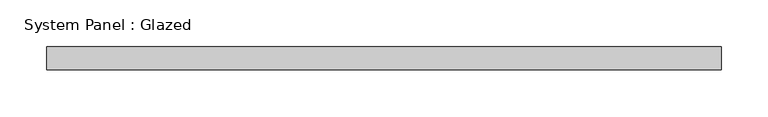
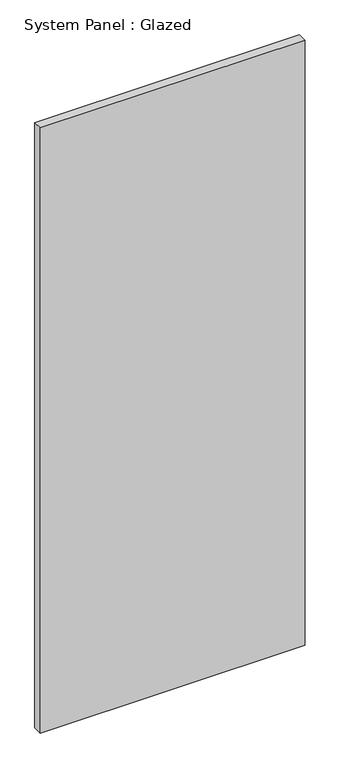
"""IFC4 building model written with IfcOpenShell, lengths in millimetres: plate geometry, System Panel : Glazed."""

from ifc_helpers import new_model, si_unit, origin, origin_with_axes, place, context, project, spatial, polyline, outline, extrude, source, transform, mapped, element, save


def system_panel_glazed_3b80f955(model_context):
    return source(origin(), model_context, "Body", "SweptSolid", [
        extrude(outline(polyline([(362.5, 24.5), (-362.5, 24.5), (-362.5, 49.5), (362.5, 49.5), (362.5, 24.5)])), origin_with_axes(), (0.0, 0.0, 1.0), 1750.0),
    ])


if __name__ == "__main__":
    model = new_model("IFC4")
    model_context = context("Model", 3, world=origin())
    ifc_project = project(units=[si_unit("LENGTHUNIT", "METRE", prefix="MILLI")], contexts=[model_context])
    site = spatial("IfcSite", under=ifc_project)
    building = spatial("IfcBuilding", under=site)
    placement = place(None, origin())
    system_panel_glazed_shape = system_panel_glazed_3b80f955(model_context)
    element("IfcPlate", 1, ObjectType="System Panel : Glazed", at=placement, inside=building, context=model_context, shape_type="MappedRepresentation", body=[
        mapped(system_panel_glazed_shape, transform((0.0, 0.0, 0.0), x_axis=(1.0, 0.0, 0.0), y_axis=(0.0, 1.0, 0.0), z_axis=(0.0, 0.0, 1.0))),
    ])
    save(model, "model.ifc")

# Revit data of these elements
# Type "System Panel : Glazed"
#   Construction Type Id = "GSP4R"
#   Analytic Construction = "1/8 in Pilkington single glazing"
#   Visual Light Transmittance = 0.9
#   Solar Heat Gain Coefficient = 0.86
#   Heat Transfer Coefficient (U) = 6.7069 W/(m²·K)
#   Define Thermal Properties by = 1
# Element 1 (IfcPlate, "System Panel : Glazed")
#   Materials on its faces: "Glass"
# Materials
#   "Glass": class "Glass", colour RGB 245 245 243, transparency 1, Description = "Soda Lime Glass", Cost = 0
